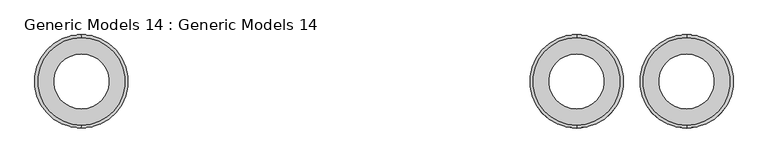
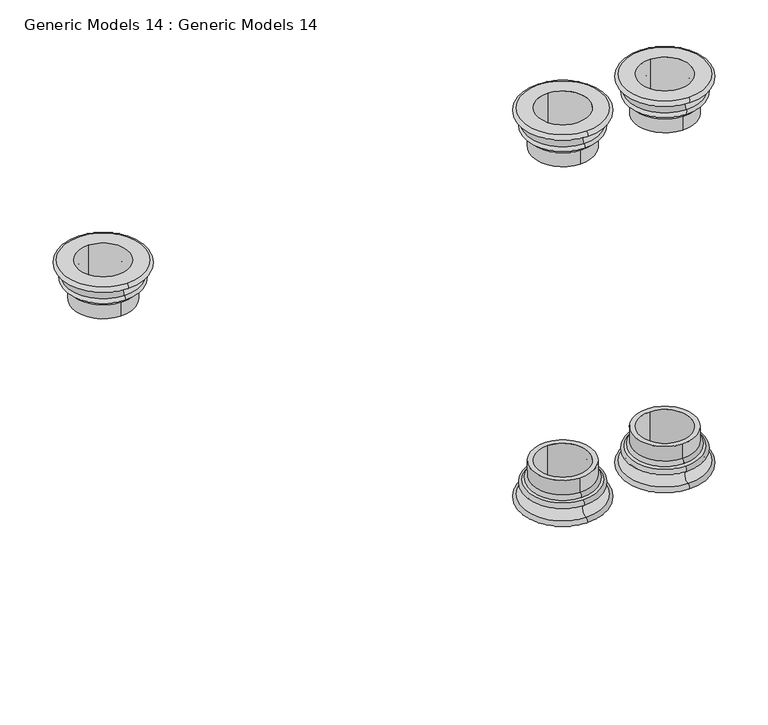
"""IFC4 building model written with IfcOpenShell, lengths in millimetres: proxy geometry, Generic Models 14 : Generic Models 14."""

from ifc_helpers import new_model, si_unit, point, frame, origin, place, context, project, spatial, polyline, circle_curve, ellipse_curve, trimmed, source, transform, mapped, element, save
from ifc_brep_helpers import plane_surface, cylinder_surface, revolved_surface, advanced_brep


def generic_models_14_generic_models_14_a82bafd3(model_context):
    return source(origin(), model_context, "Body", "AdvancedBrep", [
        advanced_brep(
        [(-2055.6825076, -7335.7292912, 2336.8), (-2055.6825076, -7742.1292912, 2336.8), (-2055.6825076, -7742.1292912, 2362.2), (-2055.6825076, -7335.7292912, 2362.2), (-2055.6825076, -7356.4126296, 2285.091654), (-2055.6825076, -7721.4459527, 2285.091654), (-2055.6825076, -7361.1292912, 2260.6), (-2055.6825076, -7716.7292912, 2260.6), (-2055.6825076, -7386.5292912, 2235.2), (-2055.6825076, -7691.3292912, 2235.2), (-2055.6825076, -7691.3292912, 2260.6), (-2055.6825076, -7386.5292912, 2260.6), (-2055.6825076, -7386.5292912, 2159.0), (-2055.6825076, -7691.3292912, 2159.0), (-2055.6825076, -7411.9292912, 2362.2), (-2055.6825076, -7665.9292912, 2362.2), (-2055.6825076, -7665.9292912, 2159.0), (-2055.6825076, -7411.9292912, 2159.0)],
        [
            (0, 1, circle_curve(frame((-2055.6825076, -7538.9292912, 2336.8), z_axis=(0.0, 0.0, 1.0), x_axis=(0.0, -1.0, 0.0)), 203.2)),
            (1, 2, circle_curve(frame((-2055.6825076, -7742.1292912, 2349.5), z_axis=(-1.0, 0.0, 0.0), x_axis=(0.0, -1.0, 0.0)), 12.7)),
            (2, 3, circle_curve(frame((-2055.6825076, -7538.9292912, 2362.2), z_axis=(0.0, 0.0, -1.0), x_axis=(0.0, -1.0, 0.0)), 203.2)),
            (3, 0, circle_curve(frame((-2055.6825076, -7335.7292912, 2349.5), z_axis=(-1.0, 0.0, 0.0), x_axis=(0.0, 1.0, 0.0)), 12.7)),
            (4, 5, circle_curve(frame((-2055.6825076, -7538.9292912, 2285.091654), z_axis=(0.0, 0.0, 1.0), x_axis=(0.0, -1.0, 0.0)), 182.5166616)),
            (5, 1, circle_curve(frame((-2055.6825076, -7742.1292912, 2306.8091593), z_axis=(1.0, 0.0, 0.0), x_axis=(0.0, -1.0, 0.0)), 29.9908407)),
            (0, 4, circle_curve(frame((-2055.6825076, -7335.7292912, 2306.8091593), z_axis=(1.0, 0.0, 0.0), x_axis=(0.0, 1.0, 0.0)), 29.9908407)),
            (6, 7, circle_curve(frame((-2055.6825076, -7538.9292912, 2260.6), z_axis=(0.0, 0.0, 1.0), x_axis=(0.0, -1.0, 0.0)), 177.8)),
            (7, 5, circle_curve(frame((-2055.6825076, -7716.7292912, 2273.3), z_axis=(-1.0, 0.0, 0.0), x_axis=(0.0, -1.0, 0.0)), 12.7)),
            (4, 6, circle_curve(frame((-2055.6825076, -7361.1292912, 2273.3), z_axis=(-1.0, 0.0, 0.0), x_axis=(0.0, 1.0, 0.0)), 12.7)),
            (8, 9, circle_curve(frame((-2055.6825076, -7538.9292912, 2235.2), z_axis=(0.0, 0.0, 1.0), x_axis=(0.0, -1.0, 0.0)), 152.4)),
            (9, 10, circle_curve(frame((-2055.6825076, -7691.3292912, 2247.9), z_axis=(-1.0, 0.0, 0.0), x_axis=(0.0, -1.0, 0.0)), 12.7)),
            (10, 11, circle_curve(frame((-2055.6825076, -7538.9292912, 2260.6), z_axis=(0.0, 0.0, -1.0), x_axis=(0.0, -1.0, 0.0)), 152.4)),
            (11, 8, circle_curve(frame((-2055.6825076, -7386.5292912, 2247.9), z_axis=(-1.0, 0.0, 0.0), x_axis=(0.0, 1.0, 0.0)), 12.7)),
            (12, 13, circle_curve(frame((-2055.6825076, -7538.9292912, 2159.0), z_axis=(0.0, 0.0, 1.0), x_axis=(0.0, -1.0, 0.0)), 152.4)),
            (13, 9),
            (8, 12),
            (14, 15, circle_curve(frame((-2055.6825076, -7538.9292912, 2362.2), z_axis=(0.0, 0.0, 1.0), x_axis=(0.0, -1.0, 0.0)), 127.0)),
            (15, 16),
            (16, 17, circle_curve(frame((-2055.6825076, -7538.9292912, 2159.0), z_axis=(0.0, 0.0, -1.0), x_axis=(0.0, -1.0, 0.0)), 127.0)),
            (17, 14),
            (1, 0, circle_curve(frame((-2055.6825076, -7538.9292912, 2336.8), z_axis=(0.0, 0.0, 1.0), x_axis=(0.0, 1.0, 0.0)), 203.2)),
            (3, 2, circle_curve(frame((-2055.6825076, -7538.9292912, 2362.2), z_axis=(0.0, 0.0, -1.0), x_axis=(0.0, 1.0, 0.0)), 203.2)),
            (5, 4, circle_curve(frame((-2055.6825076, -7538.9292912, 2285.091654), z_axis=(0.0, 0.0, 1.0), x_axis=(0.0, 1.0, 0.0)), 182.5166616)),
            (7, 6, circle_curve(frame((-2055.6825076, -7538.9292912, 2260.6), z_axis=(0.0, 0.0, 1.0), x_axis=(0.0, 1.0, 0.0)), 177.8)),
            (10, 11, circle_curve(frame((-2055.6825076, -7538.9292912, 2260.6), z_axis=(0.0, 0.0, 1.0), x_axis=(0.0, 1.0, 0.0)), 152.4)),
            (9, 8, circle_curve(frame((-2055.6825076, -7538.9292912, 2235.2), z_axis=(0.0, 0.0, 1.0), x_axis=(0.0, 1.0, 0.0)), 152.4)),
            (13, 12, circle_curve(frame((-2055.6825076, -7538.9292912, 2159.0), z_axis=(0.0, 0.0, 1.0), x_axis=(0.0, 1.0, 0.0)), 152.4)),
            (16, 17, circle_curve(frame((-2055.6825076, -7538.9292912, 2159.0), z_axis=(0.0, 0.0, 1.0), x_axis=(0.0, 1.0, 0.0)), 127.0)),
            (15, 14, circle_curve(frame((-2055.6825076, -7538.9292912, 2362.2), z_axis=(0.0, 0.0, 1.0), x_axis=(0.0, 1.0, 0.0)), 127.0)),
        ],
        [
            revolved_surface(trimmed(ellipse_curve(frame((-2055.6825076, -7742.1292912, 2349.5), z_axis=(1.0, 0.0, 0.0), x_axis=(0.0, -1.0, 0.0)), 12.7, 12.7), [point((-2055.6825076, -7742.1292912, 2362.2))], [point((-2055.6825076, -7742.1292912, 2336.8))], True, "CARTESIAN"), (-2055.6825076, -7538.9292912, 2362.2), (0.0, 0.0, -1.0)),
            revolved_surface(trimmed(ellipse_curve(frame((-2055.6825076, -7742.1292912, 2306.8091593), z_axis=(-1.0, 0.0, 0.0), x_axis=(0.0, -1.0, 0.0)), 29.9908407, 29.9908407), [point((-2055.6825076, -7742.1292912, 2336.8))], [point((-2055.6825076, -7721.4459527, 2285.091654))], True, "CARTESIAN"), (-2055.6825076, -7538.9292912, 2362.2), (0.0, 0.0, -1.0)),
            revolved_surface(trimmed(ellipse_curve(frame((-2055.6825076, -7716.7292912, 2273.3), z_axis=(1.0, 0.0, 0.0), x_axis=(0.0, -1.0, 0.0)), 12.7, 12.7), [point((-2055.6825076, -7721.4459527, 2285.091654))], [point((-2055.6825076, -7716.7292912, 2260.6))], True, "CARTESIAN"), (-2055.6825076, -7538.9292912, 2362.2), (0.0, 0.0, -1.0)),
            revolved_surface(trimmed(ellipse_curve(frame((-2055.6825076, -7691.3292912, 2247.9), z_axis=(1.0, 0.0, 0.0), x_axis=(0.0, -1.0, 0.0)), 12.7, 12.7), [point((-2055.6825076, -7691.3292912, 2260.6))], [point((-2055.6825076, -7691.3292912, 2235.2))], True, "CARTESIAN"), (-2055.6825076, -7538.9292912, 2362.2), (0.0, 0.0, -1.0)),
            cylinder_surface(frame((-2055.6825076, -7538.9292912, 2362.2), z_axis=(0.0, 0.0, -1.0), x_axis=(0.0, -1.0, 0.0)), 152.4),
            revolved_surface(polyline([(-2055.6825076, -7665.9292912, 2159.0), (-2055.6825076, -7665.9292912, 2362.2)]), (-2055.6825076, -7538.9292912, 2362.2), (0.0, 0.0, -1.0)),
            revolved_surface(trimmed(ellipse_curve(frame((-2055.6825076, -7335.7292912, 2349.5), z_axis=(-1.0, 0.0, 0.0), x_axis=(0.0, 1.0, 0.0)), 12.7, 12.7), [point((-2055.6825076, -7335.7292912, 2362.2))], [point((-2055.6825076, -7335.7292912, 2336.8))], True, "CARTESIAN"), (-2055.6825076, -7538.9292912, 2362.2), (0.0, 0.0, -1.0)),
            revolved_surface(trimmed(ellipse_curve(frame((-2055.6825076, -7335.7292912, 2306.8091593), z_axis=(1.0, 0.0, 0.0), x_axis=(0.0, 1.0, 0.0)), 29.9908407, 29.9908407), [point((-2055.6825076, -7335.7292912, 2336.8))], [point((-2055.6825076, -7356.4126296, 2285.091654))], True, "CARTESIAN"), (-2055.6825076, -7538.9292912, 2362.2), (0.0, 0.0, -1.0)),
            revolved_surface(trimmed(ellipse_curve(frame((-2055.6825076, -7361.1292912, 2273.3), z_axis=(-1.0, 0.0, 0.0), x_axis=(0.0, 1.0, 0.0)), 12.7, 12.7), [point((-2055.6825076, -7356.4126296, 2285.091654))], [point((-2055.6825076, -7361.1292912, 2260.6))], True, "CARTESIAN"), (-2055.6825076, -7538.9292912, 2362.2), (0.0, 0.0, -1.0)),
            plane_surface(frame((-2055.6825076, -7538.9292912, 2260.6), z_axis=(0.0, 0.0, -1.0), x_axis=(0.0, 1.0, 0.0))),
            revolved_surface(trimmed(ellipse_curve(frame((-2055.6825076, -7386.5292912, 2247.9), z_axis=(-1.0, 0.0, 0.0), x_axis=(0.0, 1.0, 0.0)), 12.7, 12.7), [point((-2055.6825076, -7386.5292912, 2260.6))], [point((-2055.6825076, -7386.5292912, 2235.2))], True, "CARTESIAN"), (-2055.6825076, -7538.9292912, 2362.2), (0.0, 0.0, -1.0)),
            cylinder_surface(frame((-2055.6825076, -7538.9292912, 2362.2), z_axis=(0.0, 0.0, -1.0), x_axis=(0.0, 1.0, 0.0)), 152.4),
            plane_surface(frame((-2055.6825076, -7538.9292912, 2159.0), z_axis=(0.0, 0.0, -1.0), x_axis=(0.0, 1.0, 0.0))),
            revolved_surface(polyline([(-2055.6825076, -7411.9292912, 2159.0), (-2055.6825076, -7411.9292912, 2362.2)]), (-2055.6825076, -7538.9292912, 2362.2), (0.0, 0.0, -1.0)),
            plane_surface(frame((-2055.6825076, -7538.9292912, 2362.2), z_axis=(0.0, 0.0, 1.0), x_axis=(0.0, 1.0, 0.0))),
        ],
        [
            (0, [[1, 2, 3, 4]]),
            (1, [[5, 6, -1, 7]]),
            (2, [[8, 9, -5, 10]]),
            (3, [[11, 12, 13, 14]]),
            (4, [[15, 16, -11, 17]]),
            (5, [[18, 19, 20, 21]]),
            (6, [[22, -4, 23, -2]]),
            (7, [[24, -7, -22, -6]]),
            (8, [[25, -10, -24, -9]]),
            (9, [[-25, -8], [26, -13]]),
            (10, [[27, -14, -26, -12]]),
            (11, [[28, -17, -27, -16]]),
            (12, [[-28, -15], [29, -20]]),
            (13, [[30, -21, -29, -19]]),
            (14, [[-23, -3], [-30, -18]]),
        ],
    ),
        advanced_brep(
        [(230.3174924, -7335.7292912, 2336.8), (230.3174924, -7742.1292912, 2336.8), (230.3174924, -7742.1292912, 2362.2), (230.3174924, -7335.7292912, 2362.2), (230.3174924, -7356.4126296, 2285.091654), (230.3174924, -7721.4459527, 2285.091654), (230.3174924, -7361.1292912, 2260.6), (230.3174924, -7716.7292912, 2260.6), (230.3174924, -7386.5292912, 2235.2), (230.3174924, -7691.3292912, 2235.2), (230.3174924, -7691.3292912, 2260.6), (230.3174924, -7386.5292912, 2260.6), (230.3174924, -7386.5292912, 2159.0), (230.3174924, -7691.3292912, 2159.0), (230.3174924, -7411.9292912, 2362.2), (230.3174924, -7665.9292912, 2362.2), (230.3174924, -7665.9292912, 2159.0), (230.3174924, -7411.9292912, 2159.0)],
        [
            (0, 1, circle_curve(frame((230.3174924, -7538.9292912, 2336.8), z_axis=(0.0, 0.0, 1.0), x_axis=(0.0, -1.0, 0.0)), 203.2)),
            (1, 2, circle_curve(frame((230.3174924, -7742.1292912, 2349.5), z_axis=(-1.0, 0.0, 0.0), x_axis=(0.0, -1.0, 0.0)), 12.7)),
            (2, 3, circle_curve(frame((230.3174924, -7538.9292912, 2362.2), z_axis=(0.0, 0.0, -1.0), x_axis=(0.0, -1.0, 0.0)), 203.2)),
            (3, 0, circle_curve(frame((230.3174924, -7335.7292912, 2349.5), z_axis=(-1.0, 0.0, 0.0), x_axis=(0.0, 1.0, 0.0)), 12.7)),
            (4, 5, circle_curve(frame((230.3174924, -7538.9292912, 2285.091654), z_axis=(0.0, 0.0, 1.0), x_axis=(0.0, -1.0, 0.0)), 182.5166616)),
            (5, 1, circle_curve(frame((230.3174924, -7742.1292912, 2306.8091593), z_axis=(1.0, 0.0, 0.0), x_axis=(0.0, -1.0, 0.0)), 29.9908407)),
            (0, 4, circle_curve(frame((230.3174924, -7335.7292912, 2306.8091593), z_axis=(1.0, 0.0, 0.0), x_axis=(0.0, 1.0, 0.0)), 29.9908407)),
            (6, 7, circle_curve(frame((230.3174924, -7538.9292912, 2260.6), z_axis=(0.0, 0.0, 1.0), x_axis=(0.0, -1.0, 0.0)), 177.8)),
            (7, 5, circle_curve(frame((230.3174924, -7716.7292912, 2273.3), z_axis=(-1.0, 0.0, 0.0), x_axis=(0.0, -1.0, 0.0)), 12.7)),
            (4, 6, circle_curve(frame((230.3174924, -7361.1292912, 2273.3), z_axis=(-1.0, 0.0, 0.0), x_axis=(0.0, 1.0, 0.0)), 12.7)),
            (8, 9, circle_curve(frame((230.3174924, -7538.9292912, 2235.2), z_axis=(0.0, 0.0, 1.0), x_axis=(0.0, -1.0, 0.0)), 152.4)),
            (9, 10, circle_curve(frame((230.3174924, -7691.3292912, 2247.9), z_axis=(-1.0, 0.0, 0.0), x_axis=(0.0, -1.0, 0.0)), 12.7)),
            (10, 11, circle_curve(frame((230.3174924, -7538.9292912, 2260.6), z_axis=(0.0, 0.0, -1.0), x_axis=(0.0, -1.0, 0.0)), 152.4)),
            (11, 8, circle_curve(frame((230.3174924, -7386.5292912, 2247.9), z_axis=(-1.0, 0.0, 0.0), x_axis=(0.0, 1.0, 0.0)), 12.7)),
            (12, 13, circle_curve(frame((230.3174924, -7538.9292912, 2159.0), z_axis=(0.0, 0.0, 1.0), x_axis=(0.0, -1.0, 0.0)), 152.4)),
            (13, 9),
            (8, 12),
            (14, 15, circle_curve(frame((230.3174924, -7538.9292912, 2362.2), z_axis=(0.0, 0.0, 1.0), x_axis=(0.0, -1.0, 0.0)), 127.0)),
            (15, 16),
            (16, 17, circle_curve(frame((230.3174924, -7538.9292912, 2159.0), z_axis=(0.0, 0.0, -1.0), x_axis=(0.0, -1.0, 0.0)), 127.0)),
            (17, 14),
            (1, 0, circle_curve(frame((230.3174924, -7538.9292912, 2336.8), z_axis=(0.0, 0.0, 1.0), x_axis=(0.0, 1.0, 0.0)), 203.2)),
            (3, 2, circle_curve(frame((230.3174924, -7538.9292912, 2362.2), z_axis=(0.0, 0.0, -1.0), x_axis=(0.0, 1.0, 0.0)), 203.2)),
            (5, 4, circle_curve(frame((230.3174924, -7538.9292912, 2285.091654), z_axis=(0.0, 0.0, 1.0), x_axis=(0.0, 1.0, 0.0)), 182.5166616)),
            (7, 6, circle_curve(frame((230.3174924, -7538.9292912, 2260.6), z_axis=(0.0, 0.0, 1.0), x_axis=(0.0, 1.0, 0.0)), 177.8)),
            (10, 11, circle_curve(frame((230.3174924, -7538.9292912, 2260.6), z_axis=(0.0, 0.0, 1.0), x_axis=(0.0, 1.0, 0.0)), 152.4)),
            (9, 8, circle_curve(frame((230.3174924, -7538.9292912, 2235.2), z_axis=(0.0, 0.0, 1.0), x_axis=(0.0, 1.0, 0.0)), 152.4)),
            (13, 12, circle_curve(frame((230.3174924, -7538.9292912, 2159.0), z_axis=(0.0, 0.0, 1.0), x_axis=(0.0, 1.0, 0.0)), 152.4)),
            (16, 17, circle_curve(frame((230.3174924, -7538.9292912, 2159.0), z_axis=(0.0, 0.0, 1.0), x_axis=(0.0, 1.0, 0.0)), 127.0)),
            (15, 14, circle_curve(frame((230.3174924, -7538.9292912, 2362.2), z_axis=(0.0, 0.0, 1.0), x_axis=(0.0, 1.0, 0.0)), 127.0)),
        ],
        [
            revolved_surface(trimmed(ellipse_curve(frame((230.3174924, -7742.1292912, 2349.5), z_axis=(1.0, 0.0, 0.0), x_axis=(0.0, -1.0, 0.0)), 12.7, 12.7), [point((230.3174924, -7742.1292912, 2362.2))], [point((230.3174924, -7742.1292912, 2336.8))], True, "CARTESIAN"), (230.3174924, -7538.9292912, 2362.2), (0.0, 0.0, -1.0)),
            revolved_surface(trimmed(ellipse_curve(frame((230.3174924, -7742.1292912, 2306.8091593), z_axis=(-1.0, 0.0, 0.0), x_axis=(0.0, -1.0, 0.0)), 29.9908407, 29.9908407), [point((230.3174924, -7742.1292912, 2336.8))], [point((230.3174924, -7721.4459527, 2285.091654))], True, "CARTESIAN"), (230.3174924, -7538.9292912, 2362.2), (0.0, 0.0, -1.0)),
            revolved_surface(trimmed(ellipse_curve(frame((230.3174924, -7716.7292912, 2273.3), z_axis=(1.0, 0.0, 0.0), x_axis=(0.0, -1.0, 0.0)), 12.7, 12.7), [point((230.3174924, -7721.4459527, 2285.091654))], [point((230.3174924, -7716.7292912, 2260.6))], True, "CARTESIAN"), (230.3174924, -7538.9292912, 2362.2), (0.0, 0.0, -1.0)),
            revolved_surface(trimmed(ellipse_curve(frame((230.3174924, -7691.3292912, 2247.9), z_axis=(1.0, 0.0, 0.0), x_axis=(0.0, -1.0, 0.0)), 12.7, 12.7), [point((230.3174924, -7691.3292912, 2260.6))], [point((230.3174924, -7691.3292912, 2235.2))], True, "CARTESIAN"), (230.3174924, -7538.9292912, 2362.2), (0.0, 0.0, -1.0)),
            cylinder_surface(frame((230.3174924, -7538.9292912, 2362.2), z_axis=(0.0, 0.0, -1.0), x_axis=(0.0, -1.0, 0.0)), 152.4),
            revolved_surface(polyline([(230.3174924, -7665.9292912, 2159.0), (230.3174924, -7665.9292912, 2362.2)]), (230.3174924, -7538.9292912, 2362.2), (0.0, 0.0, -1.0)),
            revolved_surface(trimmed(ellipse_curve(frame((230.3174924, -7335.7292912, 2349.5), z_axis=(-1.0, 0.0, 0.0), x_axis=(0.0, 1.0, 0.0)), 12.7, 12.7), [point((230.3174924, -7335.7292912, 2362.2))], [point((230.3174924, -7335.7292912, 2336.8))], True, "CARTESIAN"), (230.3174924, -7538.9292912, 2362.2), (0.0, 0.0, -1.0)),
            revolved_surface(trimmed(ellipse_curve(frame((230.3174924, -7335.7292912, 2306.8091593), z_axis=(1.0, 0.0, 0.0), x_axis=(0.0, 1.0, 0.0)), 29.9908407, 29.9908407), [point((230.3174924, -7335.7292912, 2336.8))], [point((230.3174924, -7356.4126296, 2285.091654))], True, "CARTESIAN"), (230.3174924, -7538.9292912, 2362.2), (0.0, 0.0, -1.0)),
            revolved_surface(trimmed(ellipse_curve(frame((230.3174924, -7361.1292912, 2273.3), z_axis=(-1.0, 0.0, 0.0), x_axis=(0.0, 1.0, 0.0)), 12.7, 12.7), [point((230.3174924, -7356.4126296, 2285.091654))], [point((230.3174924, -7361.1292912, 2260.6))], True, "CARTESIAN"), (230.3174924, -7538.9292912, 2362.2), (0.0, 0.0, -1.0)),
            plane_surface(frame((230.3174924, -7538.9292912, 2260.6), z_axis=(0.0, 0.0, -1.0), x_axis=(0.0, 1.0, 0.0))),
            revolved_surface(trimmed(ellipse_curve(frame((230.3174924, -7386.5292912, 2247.9), z_axis=(-1.0, 0.0, 0.0), x_axis=(0.0, 1.0, 0.0)), 12.7, 12.7), [point((230.3174924, -7386.5292912, 2260.6))], [point((230.3174924, -7386.5292912, 2235.2))], True, "CARTESIAN"), (230.3174924, -7538.9292912, 2362.2), (0.0, 0.0, -1.0)),
            cylinder_surface(frame((230.3174924, -7538.9292912, 2362.2), z_axis=(0.0, 0.0, -1.0), x_axis=(0.0, 1.0, 0.0)), 152.4),
            plane_surface(frame((230.3174924, -7538.9292912, 2159.0), z_axis=(0.0, 0.0, -1.0), x_axis=(0.0, 1.0, 0.0))),
            revolved_surface(polyline([(230.3174924, -7411.9292912, 2159.0), (230.3174924, -7411.9292912, 2362.2)]), (230.3174924, -7538.9292912, 2362.2), (0.0, 0.0, -1.0)),
            plane_surface(frame((230.3174924, -7538.9292912, 2362.2), z_axis=(0.0, 0.0, 1.0), x_axis=(0.0, 1.0, 0.0))),
        ],
        [
            (0, [[1, 2, 3, 4]]),
            (1, [[5, 6, -1, 7]]),
            (2, [[8, 9, -5, 10]]),
            (3, [[11, 12, 13, 14]]),
            (4, [[15, 16, -11, 17]]),
            (5, [[18, 19, 20, 21]]),
            (6, [[22, -4, 23, -2]]),
            (7, [[24, -7, -22, -6]]),
            (8, [[25, -10, -24, -9]]),
            (9, [[-25, -8], [26, -13]]),
            (10, [[27, -14, -26, -12]]),
            (11, [[28, -17, -27, -16]]),
            (12, [[-28, -15], [29, -20]]),
            (13, [[30, -21, -29, -19]]),
            (14, [[-23, -3], [-30, -18]]),
        ],
    ),
        advanced_brep(
        [(738.3174924, -7335.7292912, 2336.8), (738.3174924, -7742.1292912, 2336.8), (738.3174924, -7742.1292912, 2362.2), (738.3174924, -7335.7292912, 2362.2), (738.3174924, -7356.4126296, 2285.091654), (738.3174924, -7721.4459527, 2285.091654), (738.3174924, -7361.1292912, 2260.6), (738.3174924, -7716.7292912, 2260.6), (738.3174924, -7386.5292912, 2235.2), (738.3174924, -7691.3292912, 2235.2), (738.3174924, -7691.3292912, 2260.6), (738.3174924, -7386.5292912, 2260.6), (738.3174924, -7386.5292912, 2159.0), (738.3174924, -7691.3292912, 2159.0), (738.3174924, -7411.9292912, 2362.2), (738.3174924, -7665.9292912, 2362.2), (738.3174924, -7665.9292912, 2159.0), (738.3174924, -7411.9292912, 2159.0)],
        [
            (0, 1, circle_curve(frame((738.3174924, -7538.9292912, 2336.8), z_axis=(0.0, 0.0, 1.0), x_axis=(0.0, -1.0, 0.0)), 203.2)),
            (1, 2, circle_curve(frame((738.3174924, -7742.1292912, 2349.5), z_axis=(-1.0, 0.0, 0.0), x_axis=(0.0, -1.0, 0.0)), 12.7)),
            (2, 3, circle_curve(frame((738.3174924, -7538.9292912, 2362.2), z_axis=(0.0, 0.0, -1.0), x_axis=(0.0, -1.0, 0.0)), 203.2)),
            (3, 0, circle_curve(frame((738.3174924, -7335.7292912, 2349.5), z_axis=(-1.0, 0.0, 0.0), x_axis=(0.0, 1.0, 0.0)), 12.7)),
            (4, 5, circle_curve(frame((738.3174924, -7538.9292912, 2285.091654), z_axis=(0.0, 0.0, 1.0), x_axis=(0.0, -1.0, 0.0)), 182.5166616)),
            (5, 1, circle_curve(frame((738.3174924, -7742.1292912, 2306.8091593), z_axis=(1.0, 0.0, 0.0), x_axis=(0.0, -1.0, 0.0)), 29.9908407)),
            (0, 4, circle_curve(frame((738.3174924, -7335.7292912, 2306.8091593), z_axis=(1.0, 0.0, 0.0), x_axis=(0.0, 1.0, 0.0)), 29.9908407)),
            (6, 7, circle_curve(frame((738.3174924, -7538.9292912, 2260.6), z_axis=(0.0, 0.0, 1.0), x_axis=(0.0, -1.0, 0.0)), 177.8)),
            (7, 5, circle_curve(frame((738.3174924, -7716.7292912, 2273.3), z_axis=(-1.0, 0.0, 0.0), x_axis=(0.0, -1.0, 0.0)), 12.7)),
            (4, 6, circle_curve(frame((738.3174924, -7361.1292912, 2273.3), z_axis=(-1.0, 0.0, 0.0), x_axis=(0.0, 1.0, 0.0)), 12.7)),
            (8, 9, circle_curve(frame((738.3174924, -7538.9292912, 2235.2), z_axis=(0.0, 0.0, 1.0), x_axis=(0.0, -1.0, 0.0)), 152.4)),
            (9, 10, circle_curve(frame((738.3174924, -7691.3292912, 2247.9), z_axis=(-1.0, 0.0, 0.0), x_axis=(0.0, -1.0, 0.0)), 12.7)),
            (10, 11, circle_curve(frame((738.3174924, -7538.9292912, 2260.6), z_axis=(0.0, 0.0, -1.0), x_axis=(0.0, -1.0, 0.0)), 152.4)),
            (11, 8, circle_curve(frame((738.3174924, -7386.5292912, 2247.9), z_axis=(-1.0, 0.0, 0.0), x_axis=(0.0, 1.0, 0.0)), 12.7)),
            (12, 13, circle_curve(frame((738.3174924, -7538.9292912, 2159.0), z_axis=(0.0, 0.0, 1.0), x_axis=(0.0, -1.0, 0.0)), 152.4)),
            (13, 9),
            (8, 12),
            (14, 15, circle_curve(frame((738.3174924, -7538.9292912, 2362.2), z_axis=(0.0, 0.0, 1.0), x_axis=(0.0, -1.0, 0.0)), 127.0)),
            (15, 16),
            (16, 17, circle_curve(frame((738.3174924, -7538.9292912, 2159.0), z_axis=(0.0, 0.0, -1.0), x_axis=(0.0, -1.0, 0.0)), 127.0)),
            (17, 14),
            (1, 0, circle_curve(frame((738.3174924, -7538.9292912, 2336.8), z_axis=(0.0, 0.0, 1.0), x_axis=(0.0, 1.0, 0.0)), 203.2)),
            (3, 2, circle_curve(frame((738.3174924, -7538.9292912, 2362.2), z_axis=(0.0, 0.0, -1.0), x_axis=(0.0, 1.0, 0.0)), 203.2)),
            (5, 4, circle_curve(frame((738.3174924, -7538.9292912, 2285.091654), z_axis=(0.0, 0.0, 1.0), x_axis=(0.0, 1.0, 0.0)), 182.5166616)),
            (7, 6, circle_curve(frame((738.3174924, -7538.9292912, 2260.6), z_axis=(0.0, 0.0, 1.0), x_axis=(0.0, 1.0, 0.0)), 177.8)),
            (10, 11, circle_curve(frame((738.3174924, -7538.9292912, 2260.6), z_axis=(0.0, 0.0, 1.0), x_axis=(0.0, 1.0, 0.0)), 152.4)),
            (9, 8, circle_curve(frame((738.3174924, -7538.9292912, 2235.2), z_axis=(0.0, 0.0, 1.0), x_axis=(0.0, 1.0, 0.0)), 152.4)),
            (13, 12, circle_curve(frame((738.3174924, -7538.9292912, 2159.0), z_axis=(0.0, 0.0, 1.0), x_axis=(0.0, 1.0, 0.0)), 152.4)),
            (16, 17, circle_curve(frame((738.3174924, -7538.9292912, 2159.0), z_axis=(0.0, 0.0, 1.0), x_axis=(0.0, 1.0, 0.0)), 127.0)),
            (15, 14, circle_curve(frame((738.3174924, -7538.9292912, 2362.2), z_axis=(0.0, 0.0, 1.0), x_axis=(0.0, 1.0, 0.0)), 127.0)),
        ],
        [
            revolved_surface(trimmed(ellipse_curve(frame((738.3174924, -7742.1292912, 2349.5), z_axis=(1.0, 0.0, 0.0), x_axis=(0.0, -1.0, 0.0)), 12.7, 12.7), [point((738.3174924, -7742.1292912, 2362.2))], [point((738.3174924, -7742.1292912, 2336.8))], True, "CARTESIAN"), (738.3174924, -7538.9292912, 2362.2), (0.0, 0.0, -1.0)),
            revolved_surface(trimmed(ellipse_curve(frame((738.3174924, -7742.1292912, 2306.8091593), z_axis=(-1.0, 0.0, 0.0), x_axis=(0.0, -1.0, 0.0)), 29.9908407, 29.9908407), [point((738.3174924, -7742.1292912, 2336.8))], [point((738.3174924, -7721.4459527, 2285.091654))], True, "CARTESIAN"), (738.3174924, -7538.9292912, 2362.2), (0.0, 0.0, -1.0)),
            revolved_surface(trimmed(ellipse_curve(frame((738.3174924, -7716.7292912, 2273.3), z_axis=(1.0, 0.0, 0.0), x_axis=(0.0, -1.0, 0.0)), 12.7, 12.7), [point((738.3174924, -7721.4459527, 2285.091654))], [point((738.3174924, -7716.7292912, 2260.6))], True, "CARTESIAN"), (738.3174924, -7538.9292912, 2362.2), (0.0, 0.0, -1.0)),
            revolved_surface(trimmed(ellipse_curve(frame((738.3174924, -7691.3292912, 2247.9), z_axis=(1.0, 0.0, 0.0), x_axis=(0.0, -1.0, 0.0)), 12.7, 12.7), [point((738.3174924, -7691.3292912, 2260.6))], [point((738.3174924, -7691.3292912, 2235.2))], True, "CARTESIAN"), (738.3174924, -7538.9292912, 2362.2), (0.0, 0.0, -1.0)),
            cylinder_surface(frame((738.3174924, -7538.9292912, 2362.2), z_axis=(0.0, 0.0, -1.0), x_axis=(0.0, -1.0, 0.0)), 152.4),
            revolved_surface(polyline([(738.3174924, -7665.9292912, 2159.0), (738.3174924, -7665.9292912, 2362.2)]), (738.3174924, -7538.9292912, 2362.2), (0.0, 0.0, -1.0)),
            revolved_surface(trimmed(ellipse_curve(frame((738.3174924, -7335.7292912, 2349.5), z_axis=(-1.0, 0.0, 0.0), x_axis=(0.0, 1.0, 0.0)), 12.7, 12.7), [point((738.3174924, -7335.7292912, 2362.2))], [point((738.3174924, -7335.7292912, 2336.8))], True, "CARTESIAN"), (738.3174924, -7538.9292912, 2362.2), (0.0, 0.0, -1.0)),
            revolved_surface(trimmed(ellipse_curve(frame((738.3174924, -7335.7292912, 2306.8091593), z_axis=(1.0, 0.0, 0.0), x_axis=(0.0, 1.0, 0.0)), 29.9908407, 29.9908407), [point((738.3174924, -7335.7292912, 2336.8))], [point((738.3174924, -7356.4126296, 2285.091654))], True, "CARTESIAN"), (738.3174924, -7538.9292912, 2362.2), (0.0, 0.0, -1.0)),
            revolved_surface(trimmed(ellipse_curve(frame((738.3174924, -7361.1292912, 2273.3), z_axis=(-1.0, 0.0, 0.0), x_axis=(0.0, 1.0, 0.0)), 12.7, 12.7), [point((738.3174924, -7356.4126296, 2285.091654))], [point((738.3174924, -7361.1292912, 2260.6))], True, "CARTESIAN"), (738.3174924, -7538.9292912, 2362.2), (0.0, 0.0, -1.0)),
            plane_surface(frame((738.3174924, -7538.9292912, 2260.6), z_axis=(0.0, 0.0, -1.0), x_axis=(0.0, 1.0, 0.0))),
            revolved_surface(trimmed(ellipse_curve(frame((738.3174924, -7386.5292912, 2247.9), z_axis=(-1.0, 0.0, 0.0), x_axis=(0.0, 1.0, 0.0)), 12.7, 12.7), [point((738.3174924, -7386.5292912, 2260.6))], [point((738.3174924, -7386.5292912, 2235.2))], True, "CARTESIAN"), (738.3174924, -7538.9292912, 2362.2), (0.0, 0.0, -1.0)),
            cylinder_surface(frame((738.3174924, -7538.9292912, 2362.2), z_axis=(0.0, 0.0, -1.0), x_axis=(0.0, 1.0, 0.0)), 152.4),
            plane_surface(frame((738.3174924, -7538.9292912, 2159.0), z_axis=(0.0, 0.0, -1.0), x_axis=(0.0, 1.0, 0.0))),
            revolved_surface(polyline([(738.3174924, -7411.9292912, 2159.0), (738.3174924, -7411.9292912, 2362.2)]), (738.3174924, -7538.9292912, 2362.2), (0.0, 0.0, -1.0)),
            plane_surface(frame((738.3174924, -7538.9292912, 2362.2), z_axis=(0.0, 0.0, 1.0), x_axis=(0.0, 1.0, 0.0))),
        ],
        [
            (0, [[1, 2, 3, 4]]),
            (1, [[5, 6, -1, 7]]),
            (2, [[8, 9, -5, 10]]),
            (3, [[11, 12, 13, 14]]),
            (4, [[15, 16, -11, 17]]),
            (5, [[18, 19, 20, 21]]),
            (6, [[22, -4, 23, -2]]),
            (7, [[24, -7, -22, -6]]),
            (8, [[25, -10, -24, -9]]),
            (9, [[-25, -8], [26, -13]]),
            (10, [[27, -14, -26, -12]]),
            (11, [[28, -17, -27, -16]]),
            (12, [[-28, -15], [29, -20]]),
            (13, [[30, -21, -29, -19]]),
            (14, [[-23, -3], [-30, -18]]),
        ],
    ),
        advanced_brep(
        [(738.3174924, -7335.7292912, 330.2), (738.3174924, -7742.1292912, 330.2), (738.3174924, -7742.1292912, 304.8), (738.3174924, -7335.7292912, 304.8), (738.3174924, -7356.4126296, 381.908346), (738.3174924, -7721.4459527, 381.908346), (738.3174924, -7361.1292912, 406.4), (738.3174924, -7716.7292912, 406.4), (738.3174924, -7386.5292912, 431.8), (738.3174924, -7691.3292912, 431.8), (738.3174924, -7691.3292912, 406.4), (738.3174924, -7386.5292912, 406.4), (738.3174924, -7386.5292912, 508.0), (738.3174924, -7691.3292912, 508.0), (738.3174924, -7411.9292912, 304.8), (738.3174924, -7665.9292912, 304.8), (738.3174924, -7665.9292912, 508.0), (738.3174924, -7411.9292912, 508.0)],
        [
            (0, 1, circle_curve(frame((738.3174924, -7538.9292912, 330.2), z_axis=(0.0, 0.0, -1.0), x_axis=(0.0, -1.0, 0.0)), 203.2)),
            (1, 2, circle_curve(frame((738.3174924, -7742.1292912, 317.5), z_axis=(1.0, 0.0, 0.0), x_axis=(0.0, -1.0, 0.0)), 12.7)),
            (2, 3, circle_curve(frame((738.3174924, -7538.9292912, 304.8), z_axis=(0.0, 0.0, 1.0), x_axis=(0.0, -1.0, 0.0)), 203.2)),
            (3, 0, circle_curve(frame((738.3174924, -7335.7292912, 317.5), z_axis=(1.0, 0.0, 0.0), x_axis=(0.0, 1.0, 0.0)), 12.7)),
            (4, 5, circle_curve(frame((738.3174924, -7538.9292912, 381.908346), z_axis=(0.0, 0.0, -1.0), x_axis=(0.0, -1.0, 0.0)), 182.5166616)),
            (5, 1, circle_curve(frame((738.3174924, -7742.1292912, 360.1908407), z_axis=(-1.0, 0.0, 0.0), x_axis=(0.0, -1.0, 0.0)), 29.9908407)),
            (0, 4, circle_curve(frame((738.3174924, -7335.7292912, 360.1908407), z_axis=(-1.0, 0.0, 0.0), x_axis=(0.0, 1.0, 0.0)), 29.9908407)),
            (6, 7, circle_curve(frame((738.3174924, -7538.9292912, 406.4), z_axis=(0.0, 0.0, -1.0), x_axis=(0.0, -1.0, 0.0)), 177.8)),
            (7, 5, circle_curve(frame((738.3174924, -7716.7292912, 393.7), z_axis=(1.0, 0.0, 0.0), x_axis=(0.0, -1.0, 0.0)), 12.7)),
            (4, 6, circle_curve(frame((738.3174924, -7361.1292912, 393.7), z_axis=(1.0, 0.0, 0.0), x_axis=(0.0, 1.0, 0.0)), 12.7)),
            (8, 9, circle_curve(frame((738.3174924, -7538.9292912, 431.8), z_axis=(0.0, 0.0, -1.0), x_axis=(0.0, -1.0, 0.0)), 152.4)),
            (9, 10, circle_curve(frame((738.3174924, -7691.3292912, 419.1), z_axis=(1.0, 0.0, 0.0), x_axis=(0.0, -1.0, 0.0)), 12.7)),
            (10, 11, circle_curve(frame((738.3174924, -7538.9292912, 406.4), z_axis=(0.0, 0.0, 1.0), x_axis=(0.0, -1.0, 0.0)), 152.4)),
            (11, 8, circle_curve(frame((738.3174924, -7386.5292912, 419.1), z_axis=(1.0, 0.0, 0.0), x_axis=(0.0, 1.0, 0.0)), 12.7)),
            (12, 13, circle_curve(frame((738.3174924, -7538.9292912, 508.0), z_axis=(0.0, 0.0, -1.0), x_axis=(0.0, -1.0, 0.0)), 152.4)),
            (13, 9),
            (8, 12),
            (14, 15, circle_curve(frame((738.3174924, -7538.9292912, 304.8), z_axis=(0.0, 0.0, -1.0), x_axis=(0.0, -1.0, 0.0)), 127.0)),
            (15, 16),
            (16, 17, circle_curve(frame((738.3174924, -7538.9292912, 508.0), z_axis=(0.0, 0.0, 1.0), x_axis=(0.0, -1.0, 0.0)), 127.0)),
            (17, 14),
            (1, 0, circle_curve(frame((738.3174924, -7538.9292912, 330.2), z_axis=(0.0, 0.0, -1.0), x_axis=(0.0, 1.0, 0.0)), 203.2)),
            (3, 2, circle_curve(frame((738.3174924, -7538.9292912, 304.8), z_axis=(0.0, 0.0, 1.0), x_axis=(0.0, 1.0, 0.0)), 203.2)),
            (5, 4, circle_curve(frame((738.3174924, -7538.9292912, 381.908346), z_axis=(0.0, 0.0, -1.0), x_axis=(0.0, 1.0, 0.0)), 182.5166616)),
            (7, 6, circle_curve(frame((738.3174924, -7538.9292912, 406.4), z_axis=(0.0, 0.0, -1.0), x_axis=(0.0, 1.0, 0.0)), 177.8)),
            (10, 11, circle_curve(frame((738.3174924, -7538.9292912, 406.4), z_axis=(0.0, 0.0, -1.0), x_axis=(0.0, 1.0, 0.0)), 152.4)),
            (9, 8, circle_curve(frame((738.3174924, -7538.9292912, 431.8), z_axis=(0.0, 0.0, -1.0), x_axis=(0.0, 1.0, 0.0)), 152.4)),
            (13, 12, circle_curve(frame((738.3174924, -7538.9292912, 508.0), z_axis=(0.0, 0.0, -1.0), x_axis=(0.0, 1.0, 0.0)), 152.4)),
            (16, 17, circle_curve(frame((738.3174924, -7538.9292912, 508.0), z_axis=(0.0, 0.0, -1.0), x_axis=(0.0, 1.0, 0.0)), 127.0)),
            (15, 14, circle_curve(frame((738.3174924, -7538.9292912, 304.8), z_axis=(0.0, 0.0, -1.0), x_axis=(0.0, 1.0, 0.0)), 127.0)),
        ],
        [
            revolved_surface(trimmed(ellipse_curve(frame((738.3174924, -7742.1292912, 317.5), z_axis=(-1.0, 0.0, 0.0), x_axis=(0.0, -1.0, 0.0)), 12.7, 12.7), [point((738.3174924, -7742.1292912, 304.8))], [point((738.3174924, -7742.1292912, 330.2))], True, "CARTESIAN"), (738.3174924, -7538.9292912, 304.8), (0.0, 0.0, 1.0)),
            revolved_surface(trimmed(ellipse_curve(frame((738.3174924, -7742.1292912, 360.1908407), z_axis=(1.0, 0.0, 0.0), x_axis=(0.0, -1.0, 0.0)), 29.9908407, 29.9908407), [point((738.3174924, -7742.1292912, 330.2))], [point((738.3174924, -7721.4459527, 381.908346))], True, "CARTESIAN"), (738.3174924, -7538.9292912, 304.8), (0.0, 0.0, 1.0)),
            revolved_surface(trimmed(ellipse_curve(frame((738.3174924, -7716.7292912, 393.7), z_axis=(-1.0, 0.0, 0.0), x_axis=(0.0, -1.0, 0.0)), 12.7, 12.7), [point((738.3174924, -7721.4459527, 381.908346))], [point((738.3174924, -7716.7292912, 406.4))], True, "CARTESIAN"), (738.3174924, -7538.9292912, 304.8), (0.0, 0.0, 1.0)),
            revolved_surface(trimmed(ellipse_curve(frame((738.3174924, -7691.3292912, 419.1), z_axis=(-1.0, 0.0, 0.0), x_axis=(0.0, -1.0, 0.0)), 12.7, 12.7), [point((738.3174924, -7691.3292912, 406.4))], [point((738.3174924, -7691.3292912, 431.8))], True, "CARTESIAN"), (738.3174924, -7538.9292912, 304.8), (0.0, 0.0, 1.0)),
            cylinder_surface(frame((738.3174924, -7538.9292912, 304.8), z_axis=(0.0, 0.0, 1.0), x_axis=(0.0, -1.0, 0.0)), 152.4),
            revolved_surface(polyline([(738.3174924, -7665.9292912, 508.0), (738.3174924, -7665.9292912, 304.8)]), (738.3174924, -7538.9292912, 304.8), (0.0, 0.0, 1.0)),
            revolved_surface(trimmed(ellipse_curve(frame((738.3174924, -7335.7292912, 317.5), z_axis=(1.0, 0.0, 0.0), x_axis=(0.0, 1.0, 0.0)), 12.7, 12.7), [point((738.3174924, -7335.7292912, 304.8))], [point((738.3174924, -7335.7292912, 330.2))], True, "CARTESIAN"), (738.3174924, -7538.9292912, 304.8), (0.0, 0.0, 1.0)),
            revolved_surface(trimmed(ellipse_curve(frame((738.3174924, -7335.7292912, 360.1908407), z_axis=(-1.0, 0.0, 0.0), x_axis=(0.0, 1.0, 0.0)), 29.9908407, 29.9908407), [point((738.3174924, -7335.7292912, 330.2))], [point((738.3174924, -7356.4126296, 381.908346))], True, "CARTESIAN"), (738.3174924, -7538.9292912, 304.8), (0.0, 0.0, 1.0)),
            revolved_surface(trimmed(ellipse_curve(frame((738.3174924, -7361.1292912, 393.7), z_axis=(1.0, 0.0, 0.0), x_axis=(0.0, 1.0, 0.0)), 12.7, 12.7), [point((738.3174924, -7356.4126296, 381.908346))], [point((738.3174924, -7361.1292912, 406.4))], True, "CARTESIAN"), (738.3174924, -7538.9292912, 304.8), (0.0, 0.0, 1.0)),
            plane_surface(frame((738.3174924, -7538.9292912, 406.4), z_axis=(0.0, 0.0, 1.0), x_axis=(0.0, 1.0, 0.0))),
            revolved_surface(trimmed(ellipse_curve(frame((738.3174924, -7386.5292912, 419.1), z_axis=(1.0, 0.0, 0.0), x_axis=(0.0, 1.0, 0.0)), 12.7, 12.7), [point((738.3174924, -7386.5292912, 406.4))], [point((738.3174924, -7386.5292912, 431.8))], True, "CARTESIAN"), (738.3174924, -7538.9292912, 304.8), (0.0, 0.0, 1.0)),
            cylinder_surface(frame((738.3174924, -7538.9292912, 304.8), z_axis=(0.0, 0.0, 1.0), x_axis=(0.0, 1.0, 0.0)), 152.4),
            plane_surface(frame((738.3174924, -7538.9292912, 508.0), z_axis=(0.0, 0.0, 1.0), x_axis=(0.0, 1.0, 0.0))),
            revolved_surface(polyline([(738.3174924, -7411.9292912, 508.0), (738.3174924, -7411.9292912, 304.8)]), (738.3174924, -7538.9292912, 304.8), (0.0, 0.0, 1.0)),
            plane_surface(frame((738.3174924, -7538.9292912, 304.8), z_axis=(0.0, 0.0, -1.0), x_axis=(0.0, 1.0, 0.0))),
        ],
        [
            (0, [[1, 2, 3, 4]]),
            (1, [[5, 6, -1, 7]]),
            (2, [[8, 9, -5, 10]]),
            (3, [[11, 12, 13, 14]]),
            (4, [[15, 16, -11, 17]]),
            (5, [[18, 19, 20, 21]]),
            (6, [[22, -4, 23, -2]]),
            (7, [[24, -7, -22, -6]]),
            (8, [[25, -10, -24, -9]]),
            (9, [[-25, -8], [26, -13]]),
            (10, [[27, -14, -26, -12]]),
            (11, [[28, -17, -27, -16]]),
            (12, [[-28, -15], [29, -20]]),
            (13, [[30, -21, -29, -19]]),
            (14, [[-23, -3], [-30, -18]]),
        ],
    ),
        advanced_brep(
        [(230.3174924, -7335.7292912, 330.2), (230.3174924, -7742.1292912, 330.2), (230.3174924, -7742.1292912, 304.8), (230.3174924, -7335.7292912, 304.8), (230.3174924, -7356.4126296, 381.908346), (230.3174924, -7721.4459527, 381.908346), (230.3174924, -7361.1292912, 406.4), (230.3174924, -7716.7292912, 406.4), (230.3174924, -7386.5292912, 431.8), (230.3174924, -7691.3292912, 431.8), (230.3174924, -7691.3292912, 406.4), (230.3174924, -7386.5292912, 406.4), (230.3174924, -7386.5292912, 508.0), (230.3174924, -7691.3292912, 508.0), (230.3174924, -7411.9292912, 304.8), (230.3174924, -7665.9292912, 304.8), (230.3174924, -7665.9292912, 508.0), (230.3174924, -7411.9292912, 508.0)],
        [
            (0, 1, circle_curve(frame((230.3174924, -7538.9292912, 330.2), z_axis=(0.0, 0.0, -1.0), x_axis=(0.0, -1.0, 0.0)), 203.2)),
            (1, 2, circle_curve(frame((230.3174924, -7742.1292912, 317.5), z_axis=(1.0, 0.0, 0.0), x_axis=(0.0, -1.0, 0.0)), 12.7)),
            (2, 3, circle_curve(frame((230.3174924, -7538.9292912, 304.8), z_axis=(0.0, 0.0, 1.0), x_axis=(0.0, -1.0, 0.0)), 203.2)),
            (3, 0, circle_curve(frame((230.3174924, -7335.7292912, 317.5), z_axis=(1.0, 0.0, 0.0), x_axis=(0.0, 1.0, 0.0)), 12.7)),
            (4, 5, circle_curve(frame((230.3174924, -7538.9292912, 381.908346), z_axis=(0.0, 0.0, -1.0), x_axis=(0.0, -1.0, 0.0)), 182.5166616)),
            (5, 1, circle_curve(frame((230.3174924, -7742.1292912, 360.1908407), z_axis=(-1.0, 0.0, 0.0), x_axis=(0.0, -1.0, 0.0)), 29.9908407)),
            (0, 4, circle_curve(frame((230.3174924, -7335.7292912, 360.1908407), z_axis=(-1.0, 0.0, 0.0), x_axis=(0.0, 1.0, 0.0)), 29.9908407)),
            (6, 7, circle_curve(frame((230.3174924, -7538.9292912, 406.4), z_axis=(0.0, 0.0, -1.0), x_axis=(0.0, -1.0, 0.0)), 177.8)),
            (7, 5, circle_curve(frame((230.3174924, -7716.7292912, 393.7), z_axis=(1.0, 0.0, 0.0), x_axis=(0.0, -1.0, 0.0)), 12.7)),
            (4, 6, circle_curve(frame((230.3174924, -7361.1292912, 393.7), z_axis=(1.0, 0.0, 0.0), x_axis=(0.0, 1.0, 0.0)), 12.7)),
            (8, 9, circle_curve(frame((230.3174924, -7538.9292912, 431.8), z_axis=(0.0, 0.0, -1.0), x_axis=(0.0, -1.0, 0.0)), 152.4)),
            (9, 10, circle_curve(frame((230.3174924, -7691.3292912, 419.1), z_axis=(1.0, 0.0, 0.0), x_axis=(0.0, -1.0, 0.0)), 12.7)),
            (10, 11, circle_curve(frame((230.3174924, -7538.9292912, 406.4), z_axis=(0.0, 0.0, 1.0), x_axis=(0.0, -1.0, 0.0)), 152.4)),
            (11, 8, circle_curve(frame((230.3174924, -7386.5292912, 419.1), z_axis=(1.0, 0.0, 0.0), x_axis=(0.0, 1.0, 0.0)), 12.7)),
            (12, 13, circle_curve(frame((230.3174924, -7538.9292912, 508.0), z_axis=(0.0, 0.0, -1.0), x_axis=(0.0, -1.0, 0.0)), 152.4)),
            (13, 9),
            (8, 12),
            (14, 15, circle_curve(frame((230.3174924, -7538.9292912, 304.8), z_axis=(0.0, 0.0, -1.0), x_axis=(0.0, -1.0, 0.0)), 127.0)),
            (15, 16),
            (16, 17, circle_curve(frame((230.3174924, -7538.9292912, 508.0), z_axis=(0.0, 0.0, 1.0), x_axis=(0.0, -1.0, 0.0)), 127.0)),
            (17, 14),
            (1, 0, circle_curve(frame((230.3174924, -7538.9292912, 330.2), z_axis=(0.0, 0.0, -1.0), x_axis=(0.0, 1.0, 0.0)), 203.2)),
            (3, 2, circle_curve(frame((230.3174924, -7538.9292912, 304.8), z_axis=(0.0, 0.0, 1.0), x_axis=(0.0, 1.0, 0.0)), 203.2)),
            (5, 4, circle_curve(frame((230.3174924, -7538.9292912, 381.908346), z_axis=(0.0, 0.0, -1.0), x_axis=(0.0, 1.0, 0.0)), 182.5166616)),
            (7, 6, circle_curve(frame((230.3174924, -7538.9292912, 406.4), z_axis=(0.0, 0.0, -1.0), x_axis=(0.0, 1.0, 0.0)), 177.8)),
            (10, 11, circle_curve(frame((230.3174924, -7538.9292912, 406.4), z_axis=(0.0, 0.0, -1.0), x_axis=(0.0, 1.0, 0.0)), 152.4)),
            (9, 8, circle_curve(frame((230.3174924, -7538.9292912, 431.8), z_axis=(0.0, 0.0, -1.0), x_axis=(0.0, 1.0, 0.0)), 152.4)),
            (13, 12, circle_curve(frame((230.3174924, -7538.9292912, 508.0), z_axis=(0.0, 0.0, -1.0), x_axis=(0.0, 1.0, 0.0)), 152.4)),
            (16, 17, circle_curve(frame((230.3174924, -7538.9292912, 508.0), z_axis=(0.0, 0.0, -1.0), x_axis=(0.0, 1.0, 0.0)), 127.0)),
            (15, 14, circle_curve(frame((230.3174924, -7538.9292912, 304.8), z_axis=(0.0, 0.0, -1.0), x_axis=(0.0, 1.0, 0.0)), 127.0)),
        ],
        [
            revolved_surface(trimmed(ellipse_curve(frame((230.3174924, -7742.1292912, 317.5), z_axis=(-1.0, 0.0, 0.0), x_axis=(0.0, -1.0, 0.0)), 12.7, 12.7), [point((230.3174924, -7742.1292912, 304.8))], [point((230.3174924, -7742.1292912, 330.2))], True, "CARTESIAN"), (230.3174924, -7538.9292912, 304.8), (0.0, 0.0, 1.0)),
            revolved_surface(trimmed(ellipse_curve(frame((230.3174924, -7742.1292912, 360.1908407), z_axis=(1.0, 0.0, 0.0), x_axis=(0.0, -1.0, 0.0)), 29.9908407, 29.9908407), [point((230.3174924, -7742.1292912, 330.2))], [point((230.3174924, -7721.4459527, 381.908346))], True, "CARTESIAN"), (230.3174924, -7538.9292912, 304.8), (0.0, 0.0, 1.0)),
            revolved_surface(trimmed(ellipse_curve(frame((230.3174924, -7716.7292912, 393.7), z_axis=(-1.0, 0.0, 0.0), x_axis=(0.0, -1.0, 0.0)), 12.7, 12.7), [point((230.3174924, -7721.4459527, 381.908346))], [point((230.3174924, -7716.7292912, 406.4))], True, "CARTESIAN"), (230.3174924, -7538.9292912, 304.8), (0.0, 0.0, 1.0)),
            revolved_surface(trimmed(ellipse_curve(frame((230.3174924, -7691.3292912, 419.1), z_axis=(-1.0, 0.0, 0.0), x_axis=(0.0, -1.0, 0.0)), 12.7, 12.7), [point((230.3174924, -7691.3292912, 406.4))], [point((230.3174924, -7691.3292912, 431.8))], True, "CARTESIAN"), (230.3174924, -7538.9292912, 304.8), (0.0, 0.0, 1.0)),
            cylinder_surface(frame((230.3174924, -7538.9292912, 304.8), z_axis=(0.0, 0.0, 1.0), x_axis=(0.0, -1.0, 0.0)), 152.4),
            revolved_surface(polyline([(230.3174924, -7665.9292912, 508.0), (230.3174924, -7665.9292912, 304.8)]), (230.3174924, -7538.9292912, 304.8), (0.0, 0.0, 1.0)),
            revolved_surface(trimmed(ellipse_curve(frame((230.3174924, -7335.7292912, 317.5), z_axis=(1.0, 0.0, 0.0), x_axis=(0.0, 1.0, 0.0)), 12.7, 12.7), [point((230.3174924, -7335.7292912, 304.8))], [point((230.3174924, -7335.7292912, 330.2))], True, "CARTESIAN"), (230.3174924, -7538.9292912, 304.8), (0.0, 0.0, 1.0)),
            revolved_surface(trimmed(ellipse_curve(frame((230.3174924, -7335.7292912, 360.1908407), z_axis=(-1.0, 0.0, 0.0), x_axis=(0.0, 1.0, 0.0)), 29.9908407, 29.9908407), [point((230.3174924, -7335.7292912, 330.2))], [point((230.3174924, -7356.4126296, 381.908346))], True, "CARTESIAN"), (230.3174924, -7538.9292912, 304.8), (0.0, 0.0, 1.0)),
            revolved_surface(trimmed(ellipse_curve(frame((230.3174924, -7361.1292912, 393.7), z_axis=(1.0, 0.0, 0.0), x_axis=(0.0, 1.0, 0.0)), 12.7, 12.7), [point((230.3174924, -7356.4126296, 381.908346))], [point((230.3174924, -7361.1292912, 406.4))], True, "CARTESIAN"), (230.3174924, -7538.9292912, 304.8), (0.0, 0.0, 1.0)),
            plane_surface(frame((230.3174924, -7538.9292912, 406.4), z_axis=(0.0, 0.0, 1.0), x_axis=(0.0, 1.0, 0.0))),
            revolved_surface(trimmed(ellipse_curve(frame((230.3174924, -7386.5292912, 419.1), z_axis=(1.0, 0.0, 0.0), x_axis=(0.0, 1.0, 0.0)), 12.7, 12.7), [point((230.3174924, -7386.5292912, 406.4))], [point((230.3174924, -7386.5292912, 431.8))], True, "CARTESIAN"), (230.3174924, -7538.9292912, 304.8), (0.0, 0.0, 1.0)),
            cylinder_surface(frame((230.3174924, -7538.9292912, 304.8), z_axis=(0.0, 0.0, 1.0), x_axis=(0.0, 1.0, 0.0)), 152.4),
            plane_surface(frame((230.3174924, -7538.9292912, 508.0), z_axis=(0.0, 0.0, 1.0), x_axis=(0.0, 1.0, 0.0))),
            revolved_surface(polyline([(230.3174924, -7411.9292912, 508.0), (230.3174924, -7411.9292912, 304.8)]), (230.3174924, -7538.9292912, 304.8), (0.0, 0.0, 1.0)),
            plane_surface(frame((230.3174924, -7538.9292912, 304.8), z_axis=(0.0, 0.0, -1.0), x_axis=(0.0, 1.0, 0.0))),
        ],
        [
            (0, [[1, 2, 3, 4]]),
            (1, [[5, 6, -1, 7]]),
            (2, [[8, 9, -5, 10]]),
            (3, [[11, 12, 13, 14]]),
            (4, [[15, 16, -11, 17]]),
            (5, [[18, 19, 20, 21]]),
            (6, [[22, -4, 23, -2]]),
            (7, [[24, -7, -22, -6]]),
            (8, [[25, -10, -24, -9]]),
            (9, [[-25, -8], [26, -13]]),
            (10, [[27, -14, -26, -12]]),
            (11, [[28, -17, -27, -16]]),
            (12, [[-28, -15], [29, -20]]),
            (13, [[30, -21, -29, -19]]),
            (14, [[-23, -3], [-30, -18]]),
        ],
    ),
    ])


if __name__ == "__main__":
    model = new_model("IFC4")
    model_context = context("Model", 3, world=origin())
    ifc_project = project(units=[si_unit("LENGTHUNIT", "METRE", prefix="MILLI")], contexts=[model_context])
    site = spatial("IfcSite", under=ifc_project)
    building = spatial("IfcBuilding", under=site)
    placement = place(None, origin())
    generic_models_14_generic_models_14_shape = generic_models_14_generic_models_14_a82bafd3(model_context)
    element("IfcBuildingElementProxy", 1, Name="Generic Models 14 : Generic Models 14", ObjectType="Generic Models 14 : Generic Models 14", at=placement, inside=building, context=model_context, shape_type="MappedRepresentation", body=[
        mapped(generic_models_14_generic_models_14_shape, transform((0.0, 0.0, 0.0), x_axis=(1.0, 0.0, 0.0), y_axis=(0.0, 1.0, 0.0), z_axis=(0.0, 0.0, 1.0))),
    ])
    save(model, "model.ifc")
